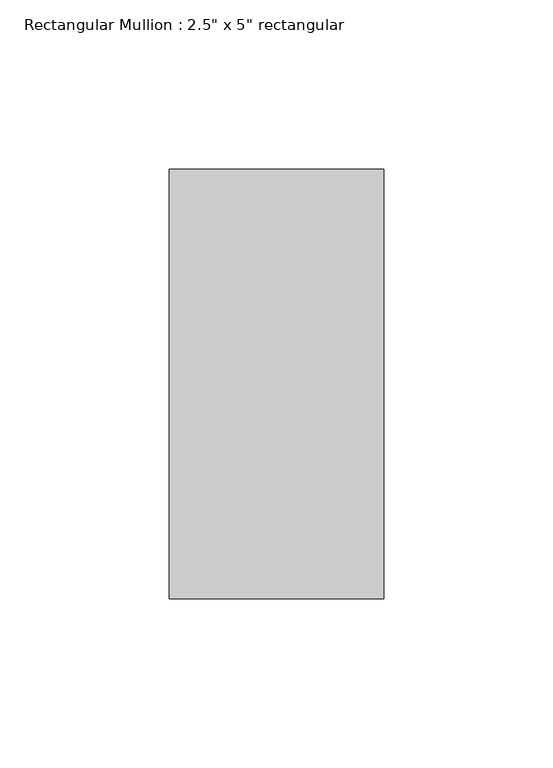
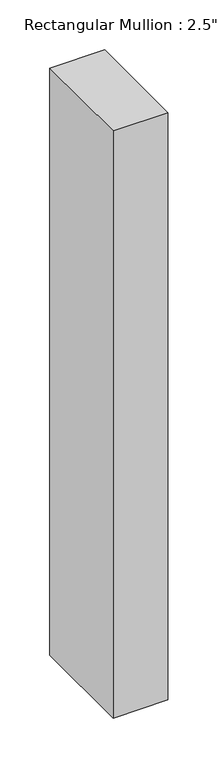
"""IFC4 building model written with IfcOpenShell, lengths in millimetres: member geometry."""

from ifc_helpers import new_model, si_unit, frame, origin, place, context, project, spatial, polyline, outline, extrude, source, transform, mapped, element, save


def member_0b2b3a95(model_context):
    return source(origin(), model_context, "Body", "SweptSolid", [
        extrude(outline(polyline([(0.0, 63.5), (0.0, -63.5), (-63.5, -63.5), (-63.5, 63.5), (0.0, 63.5)])), frame((0.0, 0.0, -719.0301467), z_axis=(0.0, 0.0, 1.0), x_axis=(1.0, 0.0, 0.0)), (0.0, 0.0, 1.0), 719.0301467),
    ])


if __name__ == "__main__":
    model = new_model("IFC4")
    model_context = context("Model", 3, world=origin())
    ifc_project = project(units=[si_unit("LENGTHUNIT", "METRE", prefix="MILLI")], contexts=[model_context])
    site = spatial("IfcSite", under=ifc_project)
    building = spatial("IfcBuilding", under=site)
    placement = place(None, origin())
    member_shape = member_0b2b3a95(model_context)
    element("IfcMember", 1, ObjectType="Rectangular Mullion : 2.5\" x 5\" rectangular", at=placement, inside=building, context=model_context, shape_type="MappedRepresentation", body=[
        mapped(member_shape, transform((0.0, 0.0, 0.0), x_axis=(1.0, 0.0, 0.0), y_axis=(0.0, 1.0, 0.0), z_axis=(0.0, 0.0, 1.0))),
    ])
    save(model, "model.ifc")

# Revit data of these elements
# Type "Rectangular Mullion : 2.5\" x 5\" rectangular"
#   built-in parameter 1007304 = 0.416667 (stored number, unit not read)
#   built-in parameter 1007301 = 0.104167 (stored number, unit not read)
#   built-in parameter 1007300 = 0.104167 (stored number, unit not read)
# Element 1 (IfcMember, "Rectangular Mullion : 2.5\" x 5\" rectangular")
#   Materials on its faces: "Aluminum"
# Materials
#   "Aluminum": class "Metal", colour RGB 247 247 247, transparency 0, Description = "Aluminum 6061", Cost = 0
